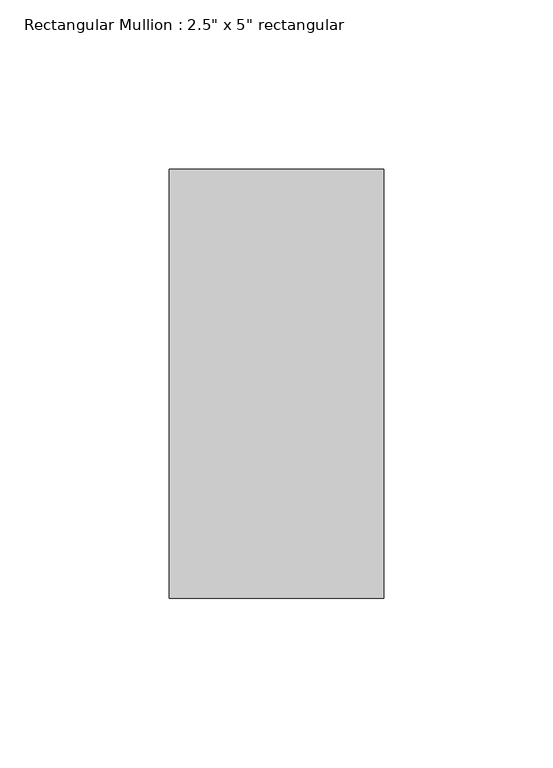
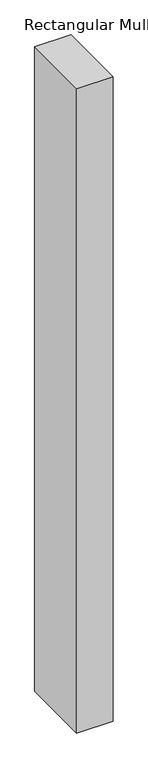
"""IFC4 building model written with IfcOpenShell, lengths in millimetres: member geometry."""

from ifc_helpers import new_model, si_unit, frame, origin, place, context, project, spatial, polyline, outline, extrude, source, transform, mapped, element, save


def member_43f7a5f1(model_context):
    return source(origin(), model_context, "Body", "SweptSolid", [
        extrude(outline(polyline([(0.0, 63.5), (0.0, -63.5), (-63.5, -63.5), (-63.5, 63.5), (0.0, 63.5)])), frame((0.0, 0.0, -1187.45), z_axis=(0.0, 0.0, 1.0), x_axis=(1.0, 0.0, 0.0)), (0.0, 0.0, 1.0), 1187.45),
    ])


if __name__ == "__main__":
    model = new_model("IFC4")
    model_context = context("Model", 3, world=origin())
    ifc_project = project(units=[si_unit("LENGTHUNIT", "METRE", prefix="MILLI")], contexts=[model_context])
    site = spatial("IfcSite", under=ifc_project)
    building = spatial("IfcBuilding", under=site)
    placement = place(None, origin())
    member_shape = member_43f7a5f1(model_context)
    element("IfcMember", 1, ObjectType="Rectangular Mullion : 2.5\" x 5\" rectangular", at=placement, inside=building, context=model_context, shape_type="MappedRepresentation", body=[
        mapped(member_shape, transform((0.0, 0.0, 0.0), x_axis=(1.0, 0.0, 0.0), y_axis=(0.0, 1.0, 0.0), z_axis=(0.0, 0.0, 1.0))),
    ])
    save(model, "model.ifc")

# Revit data of these elements
# Type "Rectangular Mullion : 2.5\" x 5\" rectangular"
#   built-in parameter 1007304 = 0.416667 (stored number, unit not read)
#   built-in parameter 1007301 = 0.104167 (stored number, unit not read)
#   built-in parameter 1007300 = 0.104167 (stored number, unit not read)
# Element 1 (IfcMember, "Rectangular Mullion : 2.5\" x 5\" rectangular")
#   Materials on its faces: "Aluminum"
# Materials
#   "Aluminum": class "Metal", colour RGB 247 247 247, transparency 0, Description = "Aluminum 6061", Cost = 0
